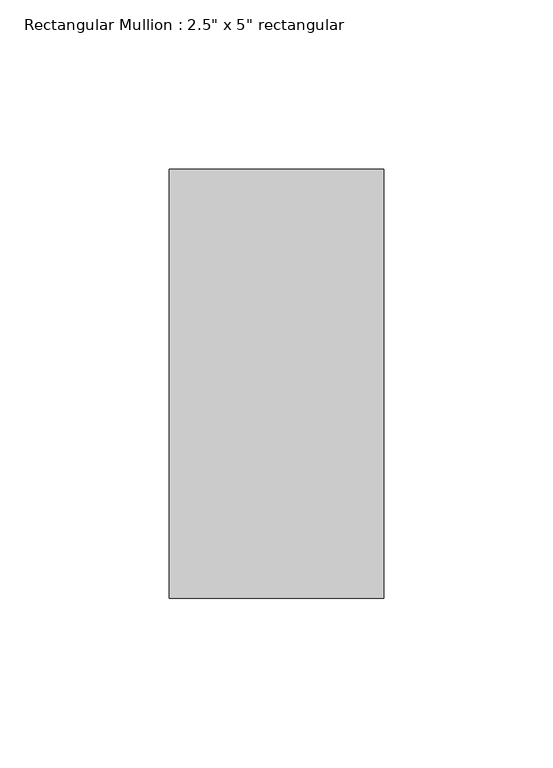
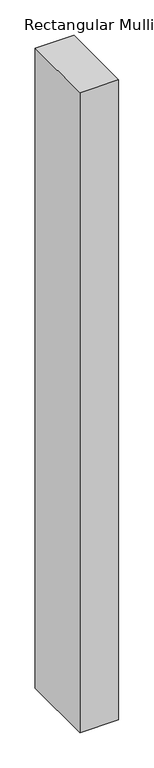
"""IFC4 building model written with IfcOpenShell, lengths in millimetres: member geometry."""

from ifc_helpers import new_model, si_unit, frame, origin, place, context, project, spatial, polyline, outline, extrude, source, transform, mapped, element, save


def member_e90b2f09(model_context):
    return source(origin(), model_context, "Body", "SweptSolid", [
        extrude(outline(polyline([(0.0, 63.5), (0.0, -63.5), (-63.5, -63.5), (-63.5, 63.5), (0.0, 63.5)])), frame((0.0, 0.0, -1106.2807647), z_axis=(0.0, 0.0, 1.0), x_axis=(1.0, 0.0, 0.0)), (0.0, 0.0, 1.0), 1106.2807647),
    ])


if __name__ == "__main__":
    model = new_model("IFC4")
    model_context = context("Model", 3, world=origin())
    ifc_project = project(units=[si_unit("LENGTHUNIT", "METRE", prefix="MILLI")], contexts=[model_context])
    site = spatial("IfcSite", under=ifc_project)
    building = spatial("IfcBuilding", under=site)
    placement = place(None, origin())
    member_shape = member_e90b2f09(model_context)
    element("IfcMember", 1, ObjectType="Rectangular Mullion : 2.5\" x 5\" rectangular", at=placement, inside=building, context=model_context, shape_type="MappedRepresentation", body=[
        mapped(member_shape, transform((0.0, 0.0, 0.0), x_axis=(1.0, 0.0, 0.0), y_axis=(0.0, 1.0, 0.0), z_axis=(0.0, 0.0, 1.0))),
    ])
    save(model, "model.ifc")

# Revit data of these elements
# Type "Rectangular Mullion : 2.5\" x 5\" rectangular"
#   built-in parameter 1007304 = 0.416667 (stored number, unit not read)
#   built-in parameter 1007301 = 0.104167 (stored number, unit not read)
#   built-in parameter 1007300 = 0.104167 (stored number, unit not read)
# Element 1 (IfcMember, "Rectangular Mullion : 2.5\" x 5\" rectangular")
#   Materials on its faces: "Aluminum"
# Materials
#   "Aluminum": class "Metal", colour RGB 247 247 247, transparency 0, Description = "Aluminum 6061", Cost = 0
